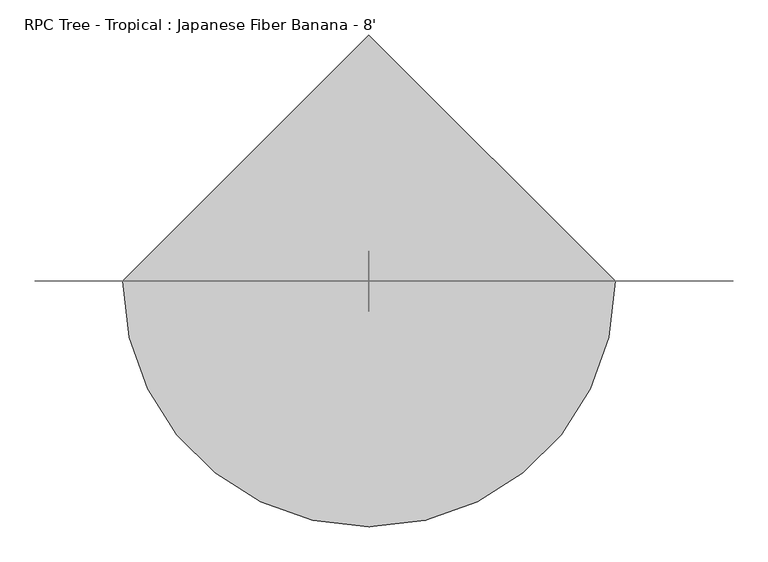
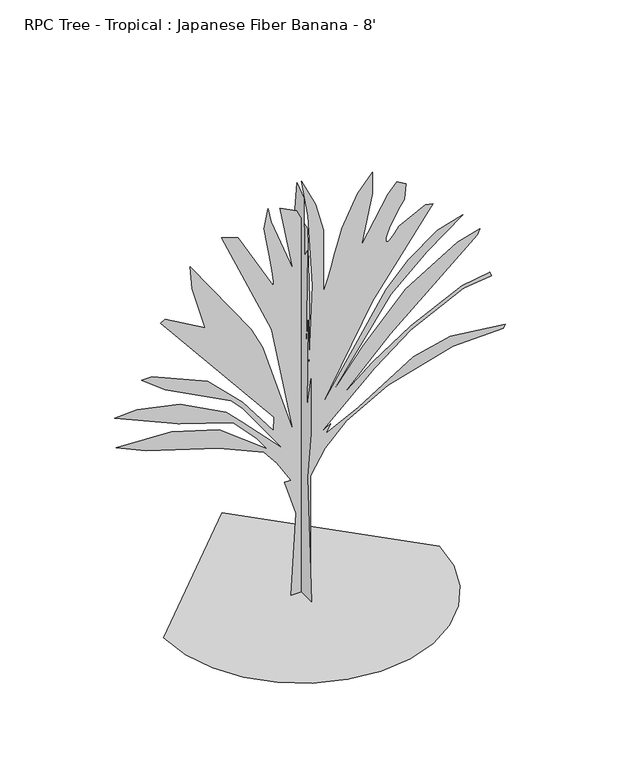
"""IFC4 building model written with IfcOpenShell, lengths in millimetres: geographic element geometry, RPC Tree - Tropical : Japanese Fiber Banana - 8'."""

from ifc_helpers import new_model, si_unit, origin, place, context, project, spatial, triangles, source, transform, mapped, element, save


def rpc_tree_tropical_japanese_fiber_banana_8_86d3d22d(model_context):
    return source(origin(), model_context, "Body", "Tessellation", [
        triangles([(-57.6944526, -0.004875, 0.0378152), (-29.4866813, -0.0049036, 479.5319581), (-95.3049203, -0.0049159, 686.3881182), (-57.6944526, -0.0049157, 683.2541525), (-136.0491993, -0.0049234, 811.7563379), (-211.2702802, -0.004929, 905.7817034), (-465.139123, -0.0049355, 1015.478496), (-872.5850378, -0.0049432, 1143.9806814), (-1041.8304485, -0.0049479, 1222.3346924), (-728.4114252, -0.0049469, 1206.6632652), (-462.0051573, -0.0049421, 1125.1752886), (-192.4648873, -0.0049298, 918.3175661), (-252.0150315, -0.0049348, 1002.9410345), (-383.6511827, -0.004943, 1140.8451897), (-690.8006395, -0.004949, 1241.1400852), (-1051.2338717, -0.0049585, 1400.9835262), (-922.7316862, -0.0049589, 1407.2530563), (-681.3987425, -0.0049557, 1353.9708435), (-424.3943716, -0.0049475, 1216.0666883), (-336.6369375, -0.0049423, 1128.3092543), (-104.7074533, -0.0049281, 890.1102762), (-327.2350405, -0.0049468, 1203.5292995), (-396.1870817, -0.004951, 1275.6169052), (-766.0222109, -0.0049626, 1469.9355675), (-897.658362, -0.0049688, 1573.36283), (-838.1082178, -0.0049688, 1573.36283), (-527.8232328, -0.0049606, 1435.4603462), (-330.3690062, -0.0049492, 1244.2740509), (-157.9880855, -0.0049354, 1012.3445303), (-154.8544287, -0.0049402, 1093.8324343), (-791.0955351, -0.0049867, 1874.2396683), (-766.0222109, -0.0049877, 1889.917345), (-540.3606943, -0.0049798, 1758.2749443), (-615.5806669, -0.0049953, 2018.4179317), (-624.9841627, -0.0050032, 2150.0603325), (-283.3563053, -0.004974, 1661.1140144), (-217.5382297, -0.0049662, 1529.4857117), (-45.1579449, -0.0049327, 968.4658133), (-167.3915631, -0.0049716, 1620.3801636), (-449.4692582, -0.0050099, 2262.8833878), (-355.4423304, -0.0050078, 2228.4174683), (-161.1236136, -0.0049871, 1880.5075996), (-156.1702277, -0.004987, 1878.9914131), (-156.8095237, -0.0049883, 1901.3121437), (-162.1099269, -0.0049909, 1943.5152363), (-171.1382639, -0.0049943, 2001.5993362), (-182.9613795, -0.0049985, 2071.6251492), (-196.6492613, -0.0050031, 2149.5914658), (-211.2702802, -0.005008, 2231.5435856), (-186.196956, -0.0050146, 2341.2403782), (-170.5255288, -0.0050097, 2259.7572704), (-48.2919151, -0.0049903, 1933.7930099), (-120.3784081, -0.0050134, 2322.4365841), (-26.352711, -0.0050106, 2275.4192505), (33.1971152, -0.005003, 2146.9186638), (45.7337819, -0.0049776, 1720.6673561), (39.4653691, -0.0049496, 1250.5419823), (61.4045732, -0.0049824, 1802.1661606), (36.3312421, -0.0050075, 2222.1495369), (1.8550919, -0.0050204, 2438.4014534), (80.2098025, -0.0050106, 2275.4192505), (124.0885286, -0.0050006, 2106.1848129), (124.0885286, -0.0049791, 1745.7390816), (127.1038605, -0.0049792, 1748.0367611), (135.5471406, -0.0049806, 1771.3891148), (148.5133368, -0.004983, 1812.2793514), (165.0985345, -0.0049863, 1867.2057953), (184.3962846, -0.0049902, 1932.6519459), (205.5040987, -0.0049945, 2005.1318241), (227.5169084, -0.0049991, 2081.0973907), (315.2743607, -0.0050095, 2256.6154564), (399.8978291, -0.0050153, 2353.7763863), (399.8978291, -0.0050078, 2228.4174683), (337.2137192, -0.0049908, 1943.2027554), (487.6552631, -0.0050056, 2190.7941833), (537.8019115, -0.0050091, 2250.347525), (587.9485963, -0.0050073, 2219.0077229), (578.5466629, -0.0050021, 2131.2565384), (555.2177453, -0.0049998, 2093.1331387), (532.9595109, -0.0049976, 2056.0412167), (512.8380283, -0.0049955, 2020.9657413), (495.9239445, -0.0049936, 1988.9383358), (483.2864528, -0.0049919, 1960.9749264), (475.9947104, -0.0049905, 1938.0757427), (475.1178017, -0.0049895, 1921.2571472), (479.3584585, -0.004989, 1912.3005718), (486.3938576, -0.004989, 1911.4096378), (495.7598193, -0.0049893, 1917.2243992), (506.9905292, -0.00499, 1928.4160126), (519.6186464, -0.0049909, 1943.640374), (533.1783566, -0.0049919, 1961.5532341), (547.2038449, -0.0049931, 1980.8103436), (697.6453526, -0.0049976, 2056.0256653), (738.3901039, -0.004997, 2046.6316166), (399.8978291, -0.0049695, 1585.8986927), (105.2834537, -0.0049378, 1053.0892817), (475.1178017, -0.0049722, 1629.7743576), (600.4860214, -0.00498, 1761.4167583), (763.4635008, -0.0049871, 1880.5075996), (907.6370407, -0.0049897, 1924.3988159), (707.0488483, -0.0049807, 1773.9526211), (503.3266903, -0.0049699, 1592.1666241), (152.2962999, -0.0049402, 1093.8324343), (349.7511443, -0.0049552, 1344.5689465), (584.8146306, -0.0049701, 1595.3084381), (876.2942591, -0.0049806, 1770.810807), (1004.7964445, -0.0049826, 1805.2922779), (989.1250174, -0.0049809, 1777.0944351), (500.1911622, -0.0049561, 1360.2387749), (227.5169084, -0.0049398, 1087.5645029), (399.8978291, -0.0049481, 1225.4686581), (616.1574486, -0.0049565, 1366.508305), (901.3675833, -0.0049647, 1504.4123875), (1061.212623, -0.0049662, 1529.4857117), (1067.4805544, -0.0049647, 1504.4123875), (910.7710791, -0.0049636, 1485.6069946), (616.1574486, -0.004955, 1341.4349808), (412.4336918, -0.0049458, 1187.8593985), (111.5518574, -0.0049292, 908.9156691), (164.8327985, -0.0049312, 943.3924891), (139.7596287, -0.0049283, 893.2442419), (321.542292, -0.0049337, 984.1356417), (628.6933113, -0.0049453, 1178.4559027), (838.6849995, -0.0049481, 1225.4686581), (1145.8360914, -0.004946, 1190.9933641), (1136.4325956, -0.0049447, 1169.0540056), (851.2209349, -0.0049443, 1162.7845482), (487.6552631, -0.004938, 1056.2232473), (252.5902508, -0.0049303, 927.7210619), (133.491225, -0.0049232, 808.6207735), (52.0021901, -0.0049152, 673.8506567), (52.0021901, -0.004875, 0.0), (0.0283614, 33.224782, 0.0319493), (0.0283545, -96.5516284, 0.0319415), (0.0283614, -60.0521984, 717.8590897), (0.0283545, -92.4963799, 997.6907009), (0.0283545, -92.4962255, 1322.1325253), (0.0283614, -55.9966365, 1127.4667912), (0.0283614, -64.1074469, 1654.6898426), (0.0283614, -43.8299509, 1464.0756054), (0.0283614, -60.0521984, 2064.2943466), (0.0283614, -31.6634243, 2015.6201374), (0.0283614, -27.6080169, 2356.2929478), (0.0283681, 41.3360625, 2404.9514603), (0.0283681, 81.8912133, 2076.4550869), (0.0283681, 94.0577399, 1606.0154881), (0.0283681, 65.6691203, 1200.4672045), (0.0283614, 33.224782, 689.4704882), (-774.8114273, 0.0, 0.0354245), (-754.3272852, -177.5359476, 0.035414), (-695.9900757, -340.5727801, 0.0354043), (-604.4718973, -484.4431409, 0.0353957), (-484.4431409, -604.4718973, 0.0353885), (-340.5727801, -695.9900757, 0.0353831), (-177.5359476, -754.3272852, 0.0353796), (2.72e-05, -774.8114273, 0.0353784), (177.5359476, -754.3272852, 0.0353796), (340.5727801, -695.9900757, 0.0353831), (484.4431409, -604.4718973, 0.0353885), (604.4718973, -484.4431409, 0.0353957), (695.9900757, -340.5727801, 0.0354043), (754.3272852, -177.5359476, 0.035414), (774.8114273, 6.77e-05, 0.0354245), (-0.0001087, 774.8114273, 0.0354708)], [[59, 60, 61], [99, 100, 101], [8, 9, 10], [49, 50, 51], [98, 99, 101], [15, 16, 17], [15, 17, 18], [119, 120, 121], [34, 35, 36], [33, 34, 36], [98, 101, 102], [97, 98, 102], [24, 25, 26], [24, 26, 27], [23, 24, 27], [23, 27, 28], [22, 23, 28], [22, 28, 29], [21, 22, 29], [7, 8, 10], [7, 10, 11], [71, 72, 73], [106, 107, 108], [106, 108, 109], [105, 106, 109], [104, 105, 109], [104, 109, 110], [103, 104, 110], [39, 40, 41], [39, 41, 42], [52, 53, 54], [52, 54, 55], [52, 55, 56], [59, 61, 62], [58, 59, 62], [58, 62, 63], [57, 58, 63], [7, 11, 12], [6, 7, 12], [15, 18, 19], [14, 15, 19], [14, 19, 20], [13, 14, 20], [13, 20, 21], [12, 13, 21], [93, 94, 95], [92, 93, 95], [91, 92, 95], [90, 91, 95], [89, 90, 95], [88, 89, 95], [87, 88, 95], [2, 3, 4], [96, 97, 102], [96, 102, 103], [124, 125, 126], [124, 126, 127], [39, 42, 43], [49, 51, 52], [48, 49, 52], [47, 48, 52], [46, 47, 52], [45, 46, 52], [44, 45, 52], [86, 87, 95], [114, 115, 116], [113, 114, 116], [30, 31, 32], [30, 32, 33], [30, 33, 36], [30, 36, 37], [30, 37, 38], [29, 30, 38], [21, 29, 38], [131, 132, 1], [131, 1, 2], [131, 2, 4], [5, 6, 12], [5, 12, 21], [123, 124, 127], [123, 127, 128], [122, 123, 128], [122, 128, 129], [121, 122, 129], [121, 129, 130], [113, 116, 117], [112, 113, 117], [111, 112, 117], [111, 117, 118], [110, 111, 118], [110, 118, 119], [103, 110, 119], [96, 103, 119], [71, 73, 74], [70, 71, 74], [69, 70, 74], [68, 69, 74], [44, 52, 56], [43, 44, 56], [39, 43, 56], [39, 56, 57], [38, 39, 57], [75, 76, 77], [75, 77, 78], [74, 75, 78], [74, 78, 79], [74, 79, 80], [74, 80, 81], [74, 81, 82], [74, 82, 83], [74, 83, 84], [74, 84, 85], [67, 68, 74], [119, 121, 130], [130, 131, 4], [130, 4, 5], [130, 5, 21], [119, 130, 21], [119, 21, 38], [96, 119, 38], [96, 38, 57], [95, 96, 57], [95, 57, 63], [95, 63, 64], [86, 95, 64], [86, 64, 65], [86, 65, 66], [86, 66, 67], [86, 67, 74], [86, 74, 85], [138, 139, 140], [136, 137, 138], [140, 141, 142], [143, 144, 145], [142, 143, 145], [142, 145, 146], [140, 142, 146], [140, 146, 147], [138, 140, 147], [138, 147, 148], [136, 138, 148], [135, 136, 148], [134, 135, 148], [134, 148, 133], [163, 164, 149], [162, 163, 149], [162, 149, 150], [161, 162, 150], [161, 150, 151], [161, 151, 152], [160, 161, 152], [159, 160, 152], [159, 152, 153], [159, 153, 154], [159, 154, 155], [159, 155, 156], [159, 156, 157], [159, 157, 158]], closed=False),
    ])


if __name__ == "__main__":
    model = new_model("IFC4")
    model_context = context("Model", 3, world=origin())
    ifc_project = project(units=[si_unit("LENGTHUNIT", "METRE", prefix="MILLI")], contexts=[model_context])
    site = spatial("IfcSite", under=ifc_project)
    building = spatial("IfcBuilding", under=site)
    placement = place(None, origin())
    rpc_tree_tropical_japanese_fiber_banana_8_shape = rpc_tree_tropical_japanese_fiber_banana_8_86d3d22d(model_context)
    element("IfcGeographicElement", 1, ObjectType="RPC Tree - Tropical : Japanese Fiber Banana - 8'", at=placement, inside=building, context=model_context, shape_type="MappedRepresentation", body=[
        mapped(rpc_tree_tropical_japanese_fiber_banana_8_shape, transform((0.0, 0.0, 0.0), x_axis=(1.0, 0.0, 0.0), y_axis=(0.0, 1.0, 0.0), z_axis=(0.0, 0.0, 1.0))),
    ])
    save(model, "model.ifc")

# Revit data of these elements
# Type "RPC Tree - Tropical : Japanese Fiber Banana - 8'"
#   built-in parameter 1005195 = "RPC-16-G2M6-EAFX-C5H6-W000-ST1L-LVER-AU"
#   Type Comments = "Japanese Fiber Banana"
#   Assembly Code = "G2050500"
#   Height = 8' - 0"
#   Plan Symbol = element 497571
#   Default Elevation = 0
